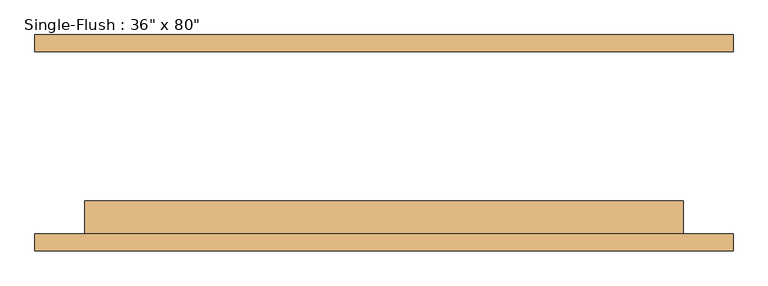
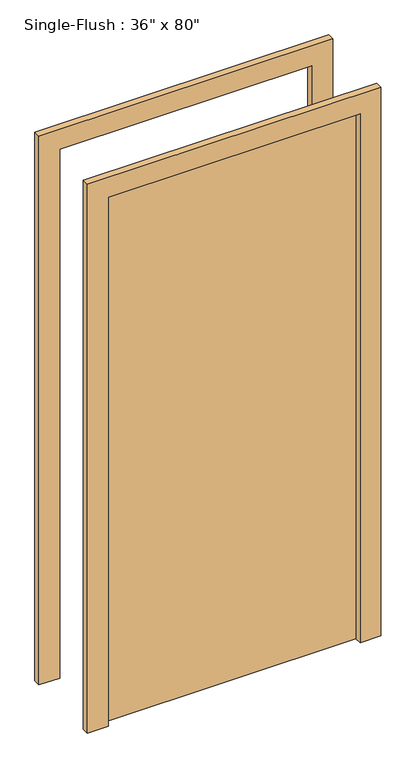
"""IFC4 building model written with IfcOpenShell, lengths in millimetres: door geometry."""

from ifc_helpers import new_model, si_unit, frame, origin, origin_with_axes, place, context, project, spatial, polyline, outline, extrude, source, transform, mapped, element, save


def door_6d3b6770(model_context):
    return source(origin(), model_context, "Body", "SweptSolid", [
        extrude(outline(polyline([(2108.2, -533.4), (0.0, -533.4), (0.0, -457.2), (2032.0, -457.2), (2032.0, 457.2), (0.0, 457.2), (0.0, 533.4), (2108.2, 533.4), (2108.2, -533.4)])), frame((0.0, -165.1, 0.0), z_axis=(0.0, 1.0, 0.0), x_axis=(0.0, 0.0, 1.0)), (0.0, 0.0, 1.0), 25.4),
        extrude(outline(polyline([(2108.2, 533.4), (2108.2, -533.4), (0.0, -533.4), (0.0, -457.2), (2032.0, -457.2), (2032.0, 457.2), (0.0, 457.2), (0.0, 533.4), (2108.2, 533.4)])), frame((0.0, 139.7, 0.0), z_axis=(0.0, 1.0, 0.0), x_axis=(0.0, 0.0, 1.0)), (0.0, 0.0, 1.0), 25.4),
        extrude(outline(polyline([(457.2, -88.9), (457.2, -139.7), (-457.2, -139.7), (-457.2, -88.9), (457.2, -88.9)])), origin_with_axes(), (0.0, 0.0, 1.0), 2032.0),
    ])


if __name__ == "__main__":
    model = new_model("IFC4")
    model_context = context("Model", 3, world=origin())
    ifc_project = project(units=[si_unit("LENGTHUNIT", "METRE", prefix="MILLI")], contexts=[model_context])
    site = spatial("IfcSite", under=ifc_project)
    building = spatial("IfcBuilding", under=site)
    placement = place(None, origin())
    door_shape = door_6d3b6770(model_context)
    element("IfcDoor", 1, ObjectType="Single-Flush : 36\" x 80\"", at=placement, inside=building, context=model_context, shape_type="MappedRepresentation", body=[
        mapped(door_shape, transform((0.0, 0.0, 0.0), x_axis=(1.0, 0.0, 0.0), y_axis=(0.0, 1.0, 0.0), z_axis=(0.0, 0.0, 1.0))),
    ])
    save(model, "model.ifc")

# Revit data of these elements
# Type "Single-Flush : 36\" x 80\""
#   Type Mark = "6"
#   Construction Type Id = "MDOOR"
#   Assembly Code = "C1020"
#   Analytic Construction = "Metal"
#   Thickness = 2"
#   Heat Transfer Coefficient (U) = 0.651978 BTU/(h·ft²·°F)
#   Height = 80"
#   Trim Projection Ext = 1"
#   Trim Projection Int = 1"
#   Trim Width = 3"
#   Width = 36"
#   Define Thermal Properties by = 1
#   Define Thermal Properties by = 1
#   Door Material = Door - Panel
#   Frame Material = Door - Frame
#   Visual Light Transmittance = 0
#   Solar Heat Gain Coefficient = 0
#   Function = (empty or 0)
#   Wall Closure = (empty or 0)
# Element 1 (IfcDoor, "Single-Flush : 36\" x 80\"")
#   Materials on its faces: "Door - Frame", "Door - Panel"
# Materials
#   "Door - Panel": class "Wood", colour RGB 210 159 95, transparency 0, Cost = 0
#   "Door - Frame": colour RGB 118 70 51, transparency 0, Cost = 0
